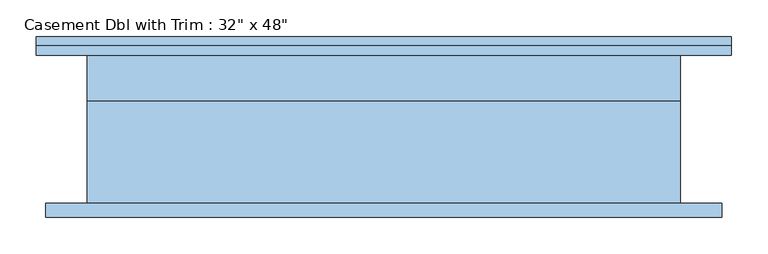
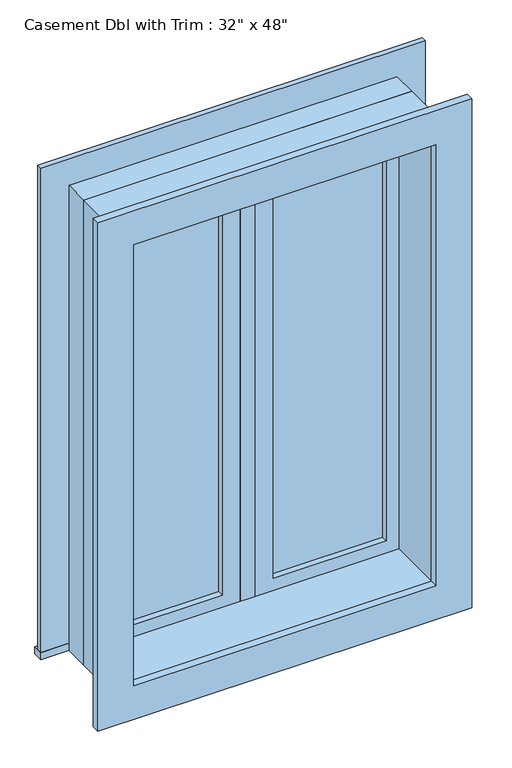
"""IFC4 building model written with IfcOpenShell, lengths in millimetres: window geometry."""

from ifc_helpers import new_model, si_unit, frame, origin, place, context, project, spatial, polyline, outline, extrude, source, transform, mapped, element, save


def window_bb17773d(model_context):
    return source(origin(), model_context, "Body", "SweptSolid", [
        extrude(outline(polyline([(63.5, 85.725), (342.9, 85.725), (342.9, 73.025), (63.5, 73.025), (63.5, 85.725)])), frame((0.0, 0.0, 977.9), z_axis=(0.0, 0.0, 1.0), x_axis=(1.0, 0.0, 0.0)), (0.0, 0.0, 1.0), 1092.2),
        extrude(outline(polyline([(2114.55, 19.05), (933.45, 19.05), (933.45, 387.35), (2114.55, 387.35), (2114.55, 19.05)]), holes=[polyline([(2070.1, 63.5), (2070.1, 342.9), (977.9, 342.9), (977.9, 63.5), (2070.1, 63.5)])]), frame((0.0, 57.15, 0.0), z_axis=(0.0, 1.0, 0.0), x_axis=(0.0, 0.0, 1.0)), (0.0, 0.0, 1.0), 44.45),
        extrude(outline(polyline([(19.05, 57.15), (-19.05, 57.15), (-19.05, 120.65), (19.05, 120.65), (19.05, 57.15)])), frame((0.0, 0.0, 933.45), z_axis=(0.0, 0.0, 1.0), x_axis=(1.0, 0.0, 0.0)), (0.0, 0.0, 1.0), 1181.1),
        extrude(outline(polyline([(-476.25, 146.05), (476.25, 146.05), (476.25, 120.65), (-476.25, 120.65), (-476.25, 146.05)])), frame((0.0, 0.0, 914.4), z_axis=(0.0, 0.0, 1.0), x_axis=(1.0, 0.0, 0.0)), (0.0, 0.0, 1.0), 19.05),
        extrude(outline(polyline([(2114.55, -387.35), (2114.55, 387.35), (933.45, 387.35), (933.45, 476.25), (2203.45, 476.25), (2203.45, -476.25), (933.45, -476.25), (933.45, -387.35), (2114.55, -387.35)])), frame((0.0, 120.65, 0.0), z_axis=(0.0, 1.0, 0.0), x_axis=(0.0, 0.0, 1.0)), (0.0, 0.0, 1.0), 12.7),
        extrude(outline(polyline([(2190.75, 463.55), (2190.75, -463.55), (857.25, -463.55), (857.25, 463.55), (2190.75, 463.55)]), holes=[polyline([(2101.85, 374.65), (946.15, 374.65), (946.15, -374.65), (2101.85, -374.65), (2101.85, 374.65)])]), frame((0.0, -101.6, 0.0), z_axis=(0.0, 1.0, 0.0), x_axis=(0.0, 0.0, 1.0)), (0.0, 0.0, 1.0), 19.05),
        extrude(outline(polyline([(-63.5, 73.025), (-342.9, 73.025), (-342.9, 85.725), (-63.5, 85.725), (-63.5, 73.025)])), frame((0.0, 0.0, 977.9), z_axis=(0.0, 0.0, 1.0), x_axis=(1.0, 0.0, 0.0)), (0.0, 0.0, 1.0), 1092.2),
        extrude(outline(polyline([(2114.55, -387.35), (933.45, -387.35), (933.45, -19.05), (2114.55, -19.05), (2114.55, -387.35)]), holes=[polyline([(2070.1, -342.9), (2070.1, -63.5), (977.9, -63.5), (977.9, -342.9), (2070.1, -342.9)])]), frame((0.0, 57.15, 0.0), z_axis=(0.0, 1.0, 0.0), x_axis=(0.0, 0.0, 1.0)), (0.0, 0.0, 1.0), 44.45),
        extrude(outline(polyline([(2133.6, -406.4), (914.4, -406.4), (914.4, 406.4), (2133.6, 406.4), (2133.6, -406.4)]), holes=[polyline([(2101.85, -374.65), (2101.85, 374.65), (946.15, 374.65), (946.15, -374.65), (2101.85, -374.65)])]), frame((0.0, -82.55, 0.0), z_axis=(0.0, 1.0, 0.0), x_axis=(0.0, 0.0, 1.0)), (0.0, 0.0, 1.0), 139.7),
        extrude(outline(polyline([(2133.6, 406.4), (2133.6, -406.4), (914.4, -406.4), (914.4, 406.4), (2133.6, 406.4)]), holes=[polyline([(2114.55, 387.35), (933.45, 387.35), (933.45, -387.35), (2114.55, -387.35), (2114.55, 387.35)])]), frame((0.0, 57.15, 0.0), z_axis=(0.0, 1.0, 0.0), x_axis=(0.0, 0.0, 1.0)), (0.0, 0.0, 1.0), 63.5),
    ])


if __name__ == "__main__":
    model = new_model("IFC4")
    model_context = context("Model", 3, world=origin())
    ifc_project = project(units=[si_unit("LENGTHUNIT", "METRE", prefix="MILLI")], contexts=[model_context])
    site = spatial("IfcSite", under=ifc_project)
    building = spatial("IfcBuilding", under=site)
    placement = place(None, origin())
    window_shape = window_bb17773d(model_context)
    element("IfcWindow", 1, ObjectType="Casement Dbl with Trim : 32\" x 48\"", at=placement, inside=building, context=model_context, shape_type="MappedRepresentation", body=[
        mapped(window_shape, transform((0.0, 0.0, 0.0), x_axis=(1.0, 0.0, 0.0), y_axis=(0.0, 1.0, 0.0), z_axis=(0.0, 0.0, 1.0))),
    ])
    save(model, "model.ifc")

# Revit data of these elements
# Type "Casement Dbl with Trim : 32\" x 48\""
#   Type Mark = "36"
#   Construction Type Id = "GSP4R"
#   Assembly Code = "B2020100"
#   Analytic Construction = "1/8 in Pilkington single glazing"
#   Visual Light Transmittance = 0.9
#   Solar Heat Gain Coefficient = 0.78
#   Heat Transfer Coefficient (U) = 0.6496 BTU/(h·ft²·°F)
#   Height = 4' - 0"
#   Default Sill Height = 3' - 0"
#   Trim Projection - Ext. = 0' - 0 1/2"
#   Trim Projection - Int. = 0' - 0 3/4"
#   Trim Width - Exterior = 0' - 3 1/2"
#   Trim Width - Interior = 0' - 3 1/2"
#   Width = 2' - 8"
#   Window Inset = 0' - 0 3/4"
#   Define Thermal Properties by = 1
#   Glass Pane Material = Glass
#   Sash Material = Sash
#   Trim Exterior Material = Trim
#   Trim Interior Material = Trim
#   Wall Closure = (empty or 0)
# Element 1 (IfcWindow, "Casement Dbl with Trim : 32\" x 48\"")
#   Materials on its faces: "Sash", "Trim", "Glass"
# Materials
#   "Glass": class "Glass", colour RGB 0 128 192, transparency 0.75, Description = "Soda Lime Glass", Cost = 0
#   "Sash": class "Wood", colour RGB 224 178 126, transparency 0
#   "Trim": class "Wood", colour RGB 224 178 126, transparency 0
